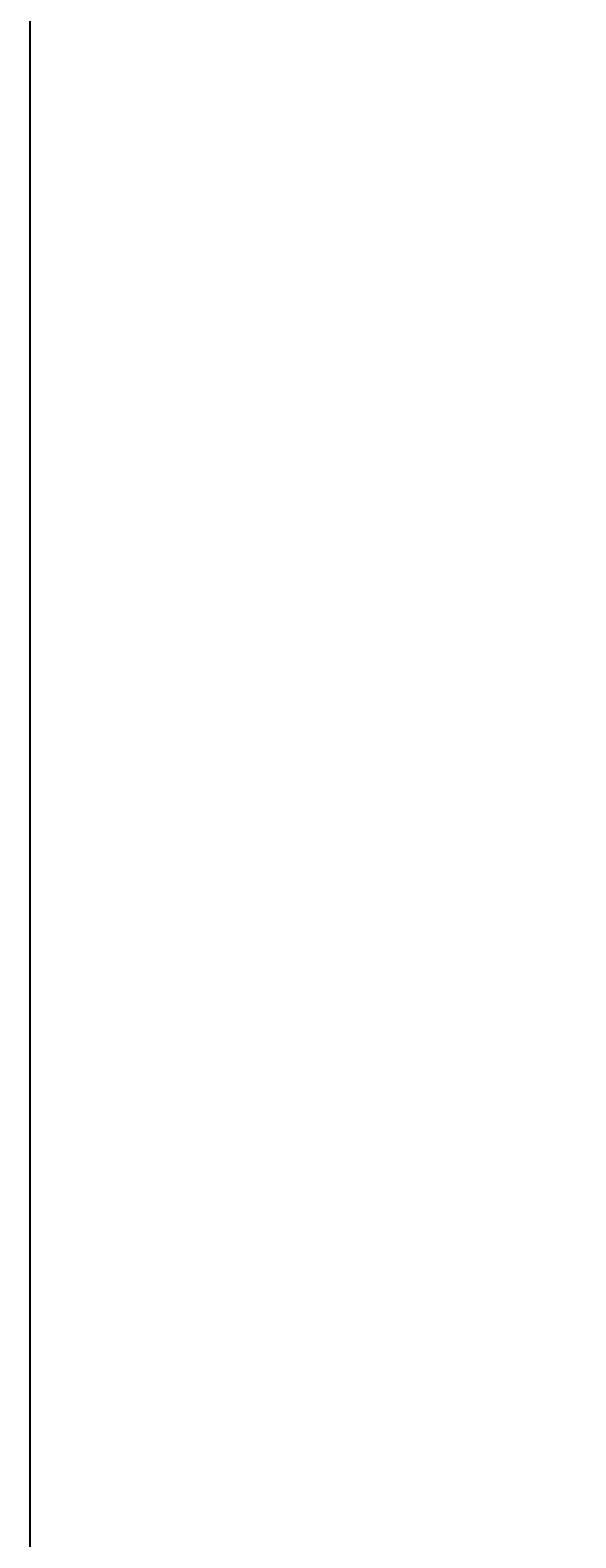
# Model space of a CAD drawing. Units: inches. Extents: x -61 to 1599, y -1316 to 257.
# Tile 126 of 204: x 372 to 388, y -166 to -122. Entities that reach past the tile are written whole.
import ezdxf

# ---------------------------------------------------------------- set-up
doc = ezdxf.new("R2010")
doc.units = ezdxf.units.IN
doc.header["$MEASUREMENT"] = 0
doc.layers.add('A-ANNO-DIMS', color=2, linetype='Continuous', lineweight=18)
doc.styles.get("Standard").update_dxf_attribs({"font": 'arial.ttf'})
doc.dimstyles.get("Standard").update_dxf_attribs({"dimtxt": 0.18, "dimasz": 0.18, "dimexe": 0.18, "dimexo": 0.0625, "dimgap": 0.09, "dimtad": 0, "dimtih": 1, "dimtoh": 1, "dimdec": 0, "dimzin": 0, "dimdsep": 46, "dimlunit": 3, "dimtxsty": 'Standard', "dimcen": 0.09, "dimadec": 0, "dimazin": 0, "dimtfac": 1, "dimtdec": 0, "dimtofl": 0, "dimtmove": 0, "dimatfit": 3, "dimfxl": 1, "dimtolj": 1, "dimtzin": 0, "dimarcsym": 0})

# ---------------------------------------------------------------- blocks, each defined once
blk = doc.blocks.new('*D703')
at = {"layer": 'A-ANNO-DIMS', "color": 0, "lineweight": -2, "transparency": 16777216}
for p, q in [((372.32, -616.882), (372.32, 257.457)), ((372.5, 257.277), (413.7, 257.277)), ((455.653, 257.277), (414.453, 257.277)), ((455.833, -616.882), (455.833, 257.457))]:
    blk.add_line(p, q, dxfattribs=at)
at = {"layer": 'A-ANNO-DIMS', "color": 0, "transparency": 16777216}
for points in [[(372.5, 257.307), (372.5, 257.247), (372.32, 257.277)], [(455.653, 257.307), (455.653, 257.247), (455.833, 257.277)]]:
    blk.add_solid(points, dxfattribs=at)
at = {"layer": 'DEFPOINTS', "color": 0, "transparency": 16777216}
for p in [(455.833, 257.277), (372.32, -616.945), (455.833, -616.945)]:
    blk.add_point(p, dxfattribs=at)
at = {"layer": 'A-ANNO-DIMS', "color": 0, "transparency": 16777216, "insert": (414.076, 257.277), "char_height": 0.18, "attachment_point": 5}
blk.add_mtext('\\A1;83.51', dxfattribs=at)

msp = doc.modelspace()

# ---------------------------------------------------------------- dimensions: what is measured, and where the dimension line sits
at = {"layer": 'A-ANNO-DIMS'}
dim = msp.add_linear_dim(base=(455.8327, 257.2771), p1=(372.3201, -616.9446), p2=(455.8327, -616.9446), dimstyle='Standard', override={"dimdec": 2, "dimlfac": 1, "dimrnd": 0, "dimzin": 0, "dimdsep": 46, "dimlunit": 2}, dxfattribs=at)
dim.commit()
dim.dimension.update_dxf_attribs({"geometry": '*D703', "text_midpoint": (414.0764, 257.2771)})

doc.saveas('drawing.dxf')
